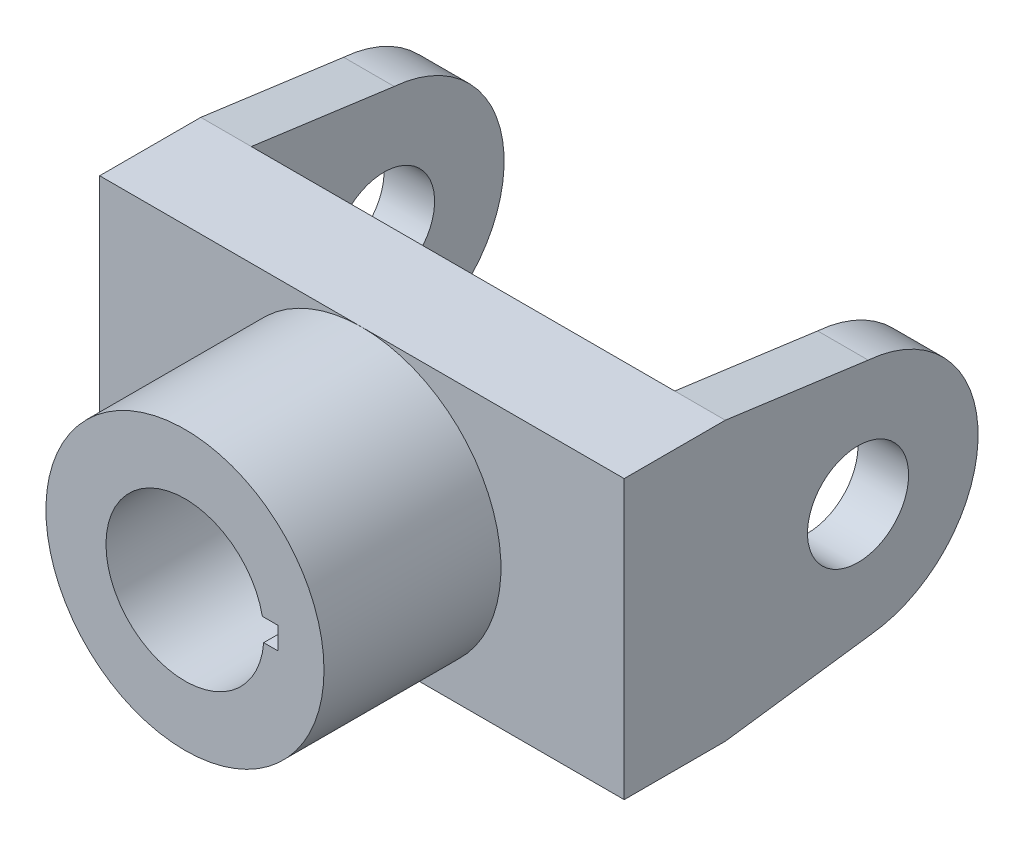
from build123d import *

# Parameters (mm, degrees)
BASE_PLATE_DEPTH    = 32
FORK_ARM_DEPTH      = 16
HUB_SKETCH_R        = 44
HUB_88_DEPTH        = 56
KEYED_BORE_50_DEPTH = 56
PIN_HOLE_SKETCH_R   = 16
PIN_HOLES_32_DEPTH  = 255


with BuildPart() as part:
    # Base Plate Sketch → Base Plate (new body)
    with BuildSketch(Plane.XY):
        Polygon((0, 0), (83, 0), (83, 88), (-83, 88), (-83, 0), align=None)
    extrude(amount=-BASE_PLATE_DEPTH)

    # Fork Arm Sketch → Fork Arm (add)
    with BuildSketch(Plane(origin=(83, 0, 0), x_dir=(0, 0, -1), z_dir=(1, 0, 0))):
        with BuildLine():
            Line((32, 88), (77.221428654, 81.863206381))
            ThreePointArc((77.221428654, 81.863206381), (111.998506035, 44.336955652), (77.892381001, 6.199876056))
            Line((77.892381001, 6.199876056), (32, 0))
            Line((32, 0), (32, 88))
        make_face()
    fork_arm = extrude(amount=-FORK_ARM_DEPTH)

    # Fork Arm Mirror: Fork Arm across plane
    add(fork_arm.mirror(Plane(origin=(0, 0, 0), x_dir=(0, 0, 1), z_dir=(1, 0, 0))))

    # Hub Sketch → Hub Ø88 (add)
    with BuildSketch(Plane.XY):
        with Locations(Location((0, 44, 0), (0, 0, 270))):
            Circle(HUB_SKETCH_R)
    extrude(amount=HUB_88_DEPTH)

    # Keyed Bore Sketch → Keyed Bore Ø50 (cut)
    with BuildSketch(Plane.XY.offset(56)):
        with BuildLine():
            Line((24.494897428, 49), (29.494897428, 49))
            Line((29.494897428, 49), (29.494897428, 42))
            Line((29.494897428, 42), (24.919871589, 42))
            ThreePointArc((24.919871589, 42), (-24.954054766, 42.485024502), (24.494897428, 49))
        make_face()
    extrude(amount=-KEYED_BORE_50_DEPTH, mode=Mode.SUBTRACT)

    # Pin Hole Sketch → Pin Holes Ø32 (cut)
    with BuildSketch(Plane(origin=(83, 0, 0), x_dir=(0, 0, -1), z_dir=(1, 0, 0))):
        with Locations(Location((74, 44, 0), (0, 0, 180))):
            Circle(PIN_HOLE_SKETCH_R)
    extrude(amount=-PIN_HOLES_32_DEPTH, mode=Mode.SUBTRACT)


solid = part.part
